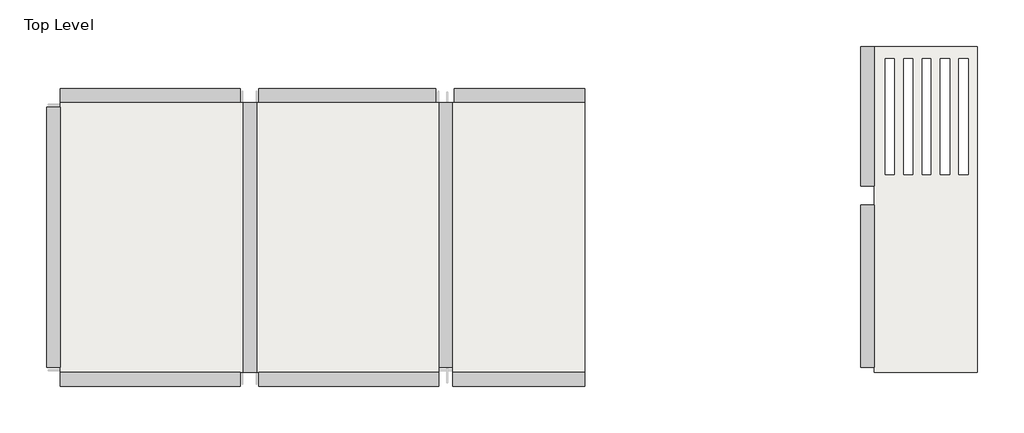
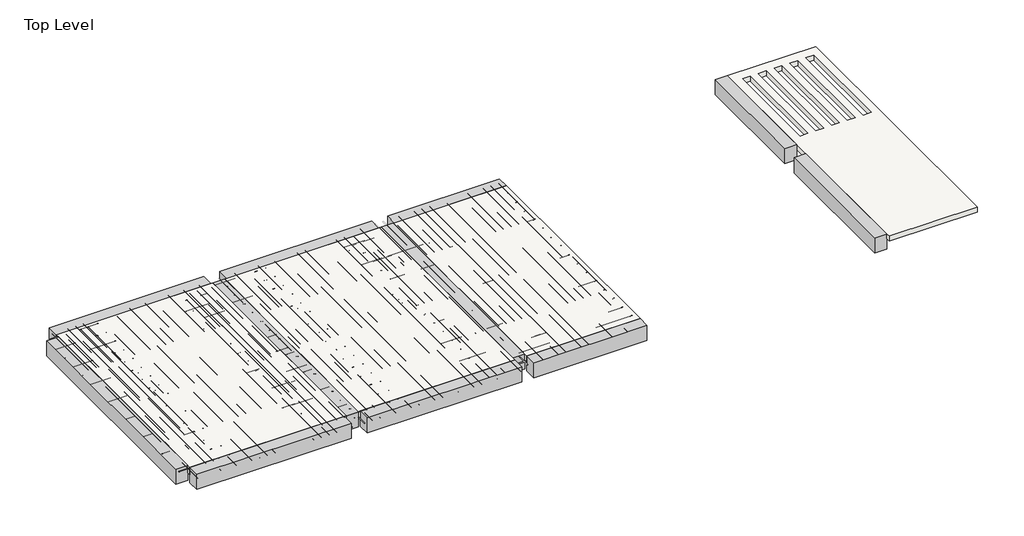
# One storey, part 1 of 2: 6 beams, 3 slabs.
"""IFC4 building model written with IfcOpenShell, lengths in millimetres."""

from ifc_helpers import new_model, si_unit, frame, origin, place, context, project, spatial, polyline, outline, extrude, faceted_brep, element, save

model = new_model("IFC4")

# Units and contexts
model_context = context("Model", 3, world=origin())
ifc_project = project(units=[si_unit("LENGTHUNIT", "METRE", prefix="MILLI")], contexts=[model_context])

# Site, building, storey
site = spatial("IfcSite", under=ifc_project)
building = spatial("IfcBuilding", under=site)
storey = spatial("IfcBuildingStorey", under=building, Name="Top Level", Elevation=12801.6)

# Beams
placement = place(None, origin())
element("IfcBeam", 1, ObjectType="M_Concrete-Rectangular Beam : 9\" X12\"", at=placement, inside=storey, context=model_context, shape_type="Brep", body=[
    faceted_brep([(-565.1117524, 415.0334631, 12801.6), (-565.1117524, 186.4334631, 12801.6), (-565.1117524, 186.4334631, 12496.8), (-565.1117524, 415.0334631, 12496.8), (-565.1117524, 415.0334631, 12649.2), (-2724.1117524, 415.0334631, 12801.6), (-2724.1117524, 186.4334631, 12801.6), (-2724.1117524, 186.4334631, 12496.8), (-2724.1117524, 415.0334631, 12496.8), (-2724.1117524, 415.0334631, 12649.2)], [[[0, 1, 2, 3, 4]], [[1, 0, 5, 6]], [[2, 1, 6, 7]], [[3, 2, 7, 8]], [[0, 4, 3, 8, 9, 5]], [[6, 5, 9, 8, 7]]]),
    faceted_brep([(-9150.3117524, 186.4334631, 12801.6), (-9150.3117524, 415.0334631, 12801.6), (-9150.3117524, 415.0334631, 12649.2), (-9150.3117524, 415.0334631, 12496.8), (-9150.3117524, 186.4334631, 12496.8), (-6203.9117524, 415.0334631, 12801.6), (-6203.9117524, 186.4334631, 12801.6), (-6203.9117524, 186.4334631, 12496.8), (-6203.9117524, 415.0334631, 12496.8)], [[[0, 1, 2, 3, 4]], [[5, 6, 7, 8]], [[1, 0, 6, 5]], [[0, 4, 7, 6]], [[4, 3, 8, 7]], [[3, 2, 1, 5, 8]]]),
    faceted_brep([(-5899.1117524, 186.4334631, 12801.6), (-5899.1117524, 415.0334631, 12801.6), (-5899.1117524, 415.0334631, 12496.8), (-5899.1117524, 186.4334631, 12496.8), (-2952.7117524, 415.0334631, 12801.6), (-2952.7117524, 186.4334631, 12801.6), (-2952.7117524, 186.4334631, 12496.8), (-2952.7117524, 415.0334631, 12496.8), (-2952.7117524, 415.0334631, 12649.2)], [[[0, 1, 2, 3]], [[4, 5, 6, 7, 8]], [[1, 0, 5, 4]], [[0, 3, 6, 5]], [[3, 2, 7, 6]], [[2, 1, 4, 8, 7]]]),
])
element("IfcBeam", 2, ObjectType="M_Concrete-Rectangular Beam : 9\" X12\"", at=placement, inside=storey, context=model_context, shape_type="Brep", body=[
    faceted_brep([(3956.0882476, 5755.7334631, 12801.6), (4184.6882476, 5755.7334631, 12801.6), (4184.6882476, 5755.7334631, 12700.0), (4184.6882476, 5755.7334631, 12496.8), (3956.0882476, 5755.7334631, 12496.8), (3956.0882476, 3463.0334631, 12801.6), (4184.6882476, 3463.0334631, 12801.6), (4184.6882476, 3463.0334631, 12496.8), (3956.0882476, 3463.0334631, 12496.8)], [[[0, 1, 2, 3, 4]], [[1, 0, 5, 6]], [[3, 2, 1, 6, 7]], [[4, 3, 7, 8]], [[0, 4, 8, 5]], [[6, 5, 8, 7]]]),
    faceted_brep([(4184.6882476, 491.2334631, 12801.6), (3956.0882476, 491.2334631, 12801.6), (3956.0882476, 491.2334631, 12496.8), (4184.6882476, 491.2334631, 12496.8), (3956.0882476, 3158.2334631, 12801.6), (4184.6882476, 3158.2334631, 12801.6), (4184.6882476, 3158.2334631, 12496.8), (3956.0882476, 3158.2334631, 12496.8)], [[[0, 1, 2, 3]], [[4, 5, 6, 7]], [[1, 0, 5, 4]], [[0, 3, 6, 5]], [[3, 2, 7, 6]], [[2, 1, 4, 7]]]),
])
element("IfcBeam", 3, ObjectType="M_Concrete-Rectangular Beam : 9\" X12\"", at=placement, inside=storey, context=model_context, shape_type="Brep", body=[
    faceted_brep([(-565.1117524, 4834.6334631, 12801.6), (-565.1117524, 4834.6334631, 12649.2), (-565.1117524, 4834.6334631, 12496.8), (-565.1117524, 5063.2334631, 12496.8), (-565.1117524, 5063.2334631, 12801.6), (-2698.7117524, 5063.2334631, 12801.6), (-2698.7117524, 5063.2334631, 12496.8), (-2698.7117524, 4834.6334631, 12496.8), (-2698.7117524, 4834.6334631, 12801.6)], [[[0, 1, 2, 3, 4]], [[5, 6, 7, 8]], [[4, 3, 6, 5]], [[0, 4, 5, 8]], [[3, 2, 7, 6]], [[2, 1, 0, 8, 7]]]),
    faceted_brep([(-3003.5117524, 4834.6334631, 12801.6), (-3003.5117524, 5063.2334631, 12801.6), (-5899.1117524, 5063.2334631, 12801.6), (-5899.1117524, 4834.6334631, 12801.6), (-3003.5117524, 5063.2334631, 12496.8), (-5899.1117524, 5063.2334631, 12496.8), (-3003.5117524, 4834.6334631, 12496.8), (-5899.1117524, 4834.6334631, 12496.8)], [[[0, 1, 2, 3]], [[1, 4, 5, 2]], [[4, 6, 7, 5]], [[6, 0, 3, 7]], [[4, 1, 0, 6]], [[3, 2, 5, 7]]]),
    faceted_brep([(-9150.3117524, 4834.6334631, 12801.6), (-9150.3117524, 5063.2334631, 12801.6), (-9150.3117524, 5063.2334631, 12496.8), (-9150.3117524, 4834.6334631, 12496.8), (-9150.3117524, 4834.6334631, 12649.2), (-6203.9117524, 5063.2334631, 12801.6), (-6203.9117524, 4834.6334631, 12801.6), (-6203.9117524, 4834.6334631, 12496.8), (-6203.9117524, 5063.2334631, 12496.8)], [[[0, 1, 2, 3, 4]], [[5, 6, 7, 8]], [[1, 0, 6, 5]], [[2, 1, 5, 8]], [[3, 2, 8, 7]], [[0, 4, 3, 7, 6]]]),
])
element("IfcBeam", 4, ObjectType="M_Concrete-Rectangular Beam : 9\" X12\"", at=placement, inside=storey, context=model_context, shape_type="SweptSolid", body=[
    extrude(outline(polyline([(-9378.9117524, 4758.4334631), (-9150.3117524, 4758.4334631), (-9150.3117524, 491.2334631), (-9378.9117524, 491.2334631), (-9378.9117524, 4758.4334631)])), frame((0.0, 0.0, 12496.8), z_axis=(0.0, 0.0, 1.0), x_axis=(1.0, 0.0, 0.0)), (0.0, 0.0, 1.0), 304.8),
])
element("IfcBeam", 5, ObjectType="M_Concrete-Rectangular Beam : 9\" X12\"", at=placement, inside=storey, context=model_context, shape_type="Brep", body=[
    faceted_brep([(-6165.8117524, 415.0334631, 12801.6), (-5937.2117524, 415.0334631, 12801.6), (-5937.2117524, 4834.6334631, 12801.6), (-6165.8117524, 4834.6334631, 12801.6), (-5937.2117524, 415.0334631, 12649.2), (-5937.2117524, 415.0334631, 12496.8), (-5937.2117524, 4834.6334631, 12496.8), (-5937.2117524, 4834.6334631, 12649.2), (-6165.8117524, 415.0334631, 12496.8), (-6165.8117524, 4834.6334631, 12496.8), (-6165.8117524, 415.0334631, 12649.2), (-6165.8117524, 4834.6334631, 12649.2)], [[[0, 1, 2, 3]], [[1, 4, 5, 6, 7, 2]], [[5, 8, 9, 6]], [[8, 10, 0, 3, 11, 9]], [[1, 0, 10, 8, 5, 4]], [[3, 2, 7, 6, 9, 11]]]),
])
element("IfcBeam", 6, ObjectType="M_Concrete-Rectangular Beam : 9\" X12\"", at=placement, inside=storey, context=model_context, shape_type="Brep", body=[
    faceted_brep([(-2952.7117524, 491.2334631, 12801.6), (-2724.1117524, 491.2334631, 12801.6), (-2724.1117524, 4834.6334631, 12801.6), (-2952.7117524, 4834.6334631, 12801.6), (-2724.1117524, 491.2334631, 12649.2), (-2724.1117524, 491.2334631, 12496.8), (-2724.1117524, 4834.6334631, 12496.8), (-2724.1117524, 4834.6334631, 12649.2), (-2952.7117524, 491.2334631, 12496.8), (-2952.7117524, 4834.6334631, 12496.8), (-2952.7117524, 4834.6334631, 12649.2), (-2952.7117524, 491.2334631, 12649.2)], [[[0, 1, 2, 3]], [[2, 1, 4, 5, 6, 7]], [[5, 8, 9, 6]], [[0, 3, 10, 9, 8, 11]], [[1, 0, 11, 8, 5, 4]], [[3, 2, 7, 6, 9, 10]]]),
])

# Slabs
element("IfcSlab", 7, ObjectType="FLOOR SLAB 6\"", at=placement, inside=storey, context=model_context, shape_type="Brep", body=[
    faceted_brep([(-6165.8117524, 4834.6334631, 12649.2), (-6165.8117524, 415.0334631, 12649.2), (-9150.3117524, 415.0334631, 12649.2), (-9150.3117524, 4834.6334631, 12649.2), (-6165.8117524, 4834.6334631, 12801.6), (-6203.9117524, 4834.6334631, 12801.6), (-9150.3117524, 4834.6334631, 12801.6), (-9150.3117524, 4758.4334631, 12801.6), (-9150.3117524, 491.2334631, 12801.6), (-9150.3117524, 415.0334631, 12801.6), (-6203.9117524, 415.0334631, 12801.6), (-6165.8117524, 415.0334631, 12801.6)], [[[0, 1, 2, 3]], [[4, 5, 6, 7, 8, 9, 10, 11]], [[1, 0, 4, 11]], [[2, 1, 11, 10, 9]], [[3, 2, 9, 8, 7, 6]], [[0, 3, 6, 5, 4]]]),
])
element("IfcSlab", 8, ObjectType="FLOOR SLAB 6\"", at=placement, inside=storey, context=model_context, shape_type="Brep", body=[
    faceted_brep([(-2952.7117524, 4834.6334631, 12649.2), (-2952.7117524, 415.0334631, 12649.2), (-5937.2117524, 415.0334631, 12649.2), (-5937.2117524, 4834.6334631, 12649.2), (-2952.7117524, 4834.6334631, 12801.6), (-3003.5117524, 4834.6334631, 12801.6), (-5899.1117524, 4834.6334631, 12801.6), (-5937.2117524, 4834.6334631, 12801.6), (-5937.2117524, 415.0334631, 12801.6), (-5899.1117524, 415.0334631, 12801.6), (-2952.7117524, 415.0334631, 12801.6), (-2952.7117524, 491.2334631, 12801.6)], [[[0, 1, 2, 3]], [[4, 5, 6, 7, 8, 9, 10, 11]], [[1, 0, 4, 11, 10]], [[2, 1, 10, 9, 8]], [[3, 2, 8, 7]], [[0, 3, 7, 6, 5, 4]]]),
    faceted_brep([(-565.1117524, 4834.6334631, 12649.2), (-565.1117524, 415.0334631, 12649.2), (-2724.1117524, 415.0334631, 12649.2), (-2724.1117524, 4834.6334631, 12649.2), (-565.1117524, 4834.6334631, 12801.6), (-2698.7117524, 4834.6334631, 12801.6), (-2724.1117524, 4834.6334631, 12801.6), (-2724.1117524, 491.2334631, 12801.6), (-2724.1117524, 415.0334631, 12801.6), (-565.1117524, 415.0334631, 12801.6)], [[[0, 1, 2, 3]], [[4, 5, 6, 7, 8, 9]], [[1, 0, 4, 9]], [[2, 1, 9, 8]], [[3, 2, 8, 7, 6]], [[0, 3, 6, 5, 4]]]),
])
element("IfcSlab", 9, ObjectType="STAIR TOWER", at=placement, inside=storey, context=model_context, shape_type="Brep", body=[
    faceted_brep([(4184.6882476, 415.0334631, 12700.0), (4184.6882476, 5755.7334631, 12700.0), (5871.6882476, 5755.7334631, 12700.0), (5871.6882476, 415.0334631, 12700.0), (4509.4989887, 5554.644792, 12700.0), (4357.0989887, 5554.644792, 12700.0), (4357.0989887, 3654.644792, 12700.0), (4509.4989887, 3654.644792, 12700.0), (4814.2989887, 5554.644792, 12700.0), (4661.8989887, 5554.644792, 12700.0), (4661.8989887, 3654.644792, 12700.0), (4814.2989887, 3654.644792, 12700.0), (5109.4989887, 5554.644792, 12700.0), (4966.6989887, 5554.644792, 12700.0), (4966.6989887, 3654.644792, 12700.0), (5109.4989887, 3654.644792, 12700.0), (5414.2989887, 5554.644792, 12700.0), (5261.8989887, 5554.644792, 12700.0), (5261.8989887, 3654.644792, 12700.0), (5414.2989887, 3654.644792, 12700.0), (5719.0989887, 5554.644792, 12700.0), (5566.6989887, 5554.644792, 12700.0), (5566.6989887, 3654.644792, 12700.0), (5719.0989887, 3654.644792, 12700.0), (4184.6882476, 415.0334631, 12801.6), (5871.6882476, 415.0334631, 12801.6), (5871.6882476, 5755.7334631, 12801.6), (4184.6882476, 5755.7334631, 12801.6), (4184.6882476, 3463.0334631, 12801.6), (4184.6882476, 3158.2334631, 12801.6), (4184.6882476, 491.2334631, 12801.6), (4509.4989887, 5554.644792, 12801.6), (4509.4989887, 3654.644792, 12801.6), (4357.0989887, 3654.644792, 12801.6), (4357.0989887, 5554.644792, 12801.6), (4814.2989887, 5554.644792, 12801.6), (4814.2989887, 3654.644792, 12801.6), (4661.8989887, 3654.644792, 12801.6), (4661.8989887, 5554.644792, 12801.6), (5109.4989887, 5554.644792, 12801.6), (5109.4989887, 3654.644792, 12801.6), (4966.6989887, 3654.644792, 12801.6), (4966.6989887, 5554.644792, 12801.6), (5414.2989887, 5554.644792, 12801.6), (5414.2989887, 3654.644792, 12801.6), (5261.8989887, 3654.644792, 12801.6), (5261.8989887, 5554.644792, 12801.6), (5719.0989887, 5554.644792, 12801.6), (5719.0989887, 3654.644792, 12801.6), (5566.6989887, 3654.644792, 12801.6), (5566.6989887, 5554.644792, 12801.6)], [[[0, 1, 2, 3], [4, 5, 6, 7], [8, 9, 10, 11], [12, 13, 14, 15], [16, 17, 18, 19], [20, 21, 22, 23]], [[24, 25, 26, 27, 28, 29, 30], [31, 32, 33, 34], [35, 36, 37, 38], [39, 40, 41, 42], [43, 44, 45, 46], [47, 48, 49, 50]], [[1, 0, 24, 30, 29, 28, 27]], [[2, 1, 27, 26]], [[3, 2, 26, 25]], [[0, 3, 25, 24]], [[5, 4, 31, 34]], [[6, 5, 34, 33]], [[7, 6, 33, 32]], [[4, 7, 32, 31]], [[9, 8, 35, 38]], [[10, 9, 38, 37]], [[11, 10, 37, 36]], [[8, 11, 36, 35]], [[13, 12, 39, 42]], [[14, 13, 42, 41]], [[15, 14, 41, 40]], [[12, 15, 40, 39]], [[17, 16, 43, 46]], [[18, 17, 46, 45]], [[19, 18, 45, 44]], [[16, 19, 44, 43]], [[21, 20, 47, 50]], [[22, 21, 50, 49]], [[23, 22, 49, 48]], [[20, 23, 48, 47]]]),
])

save(model, "model.ifc")

# Revit data of these elements
# Type "M_Concrete-Rectangular Beam : 9\" X12\""
#   Length [instance default] = 5' - 0"
#   b = 0' - 9"
#   h = 1' - 0"
#   Structural Material [instance default] = Concrete, Cast-in-Place gray
#   Assembly Code = ""
# Type "FLOOR SLAB 6\""
#   Layers, outside or top first: 0' - 6" "Concrete, Cast-in-Place gray" (function 1)
# Type "STAIR TOWER"
#   Layers, outside or top first: 0' - 4" "Concrete, Cast-in-Place gray" (function 1)
# Elements 1, 2, 3, 4, 5, 6 (IfcBeam, "M_Concrete-Rectangular Beam : 9\" X12\"")
#   Structural Material = Concrete, Cast-in-Place gray
#   Phase Created = New Construction
#   Materials on its faces: "Concrete, Cast-in-Place gray"
# Elements 7, 8 (IfcSlab, "FLOOR SLAB 6\"")
#   Height Offset From Level = 0' - 0"
#   built-in parameter 1001954 = 1
#   Phase Created = New Construction
#   Materials on its faces: "Concrete, Cast-in-Place gray"
# Element 9 (IfcSlab, "STAIR TOWER")
#   built-in parameter 1001955 = 3.14159 (stored number, unit not read)
#   Height Offset From Level = 0' - 0"
#   built-in parameter 1001954 = 1
#   Phase Created = New Construction
#   Materials on its faces: "Concrete, Cast-in-Place gray"
# Materials
#   "Concrete, Cast-in-Place gray": class "Concrete", colour RGB 192 192 192, transparency 0, Description = "Cast-in-place concrete", Cost = 0
